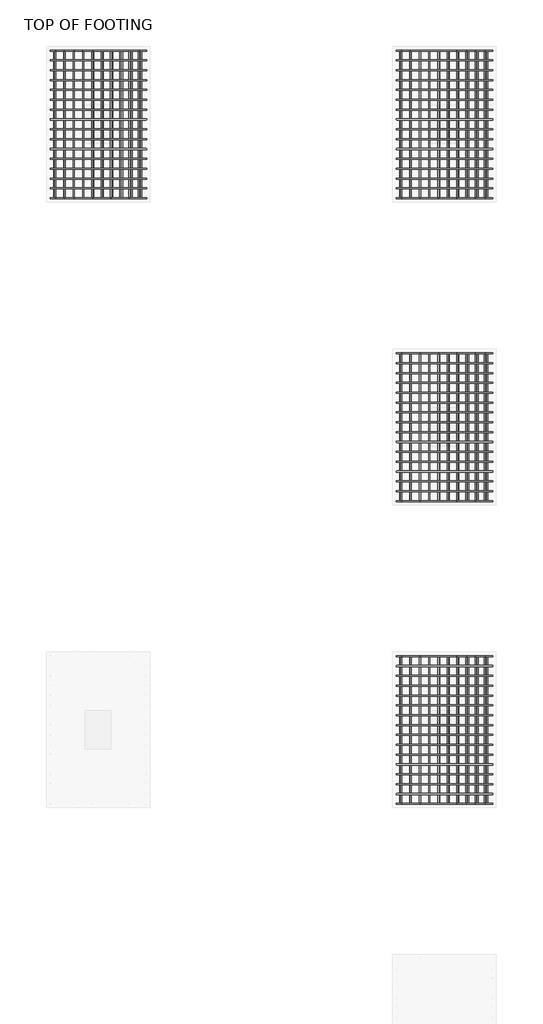
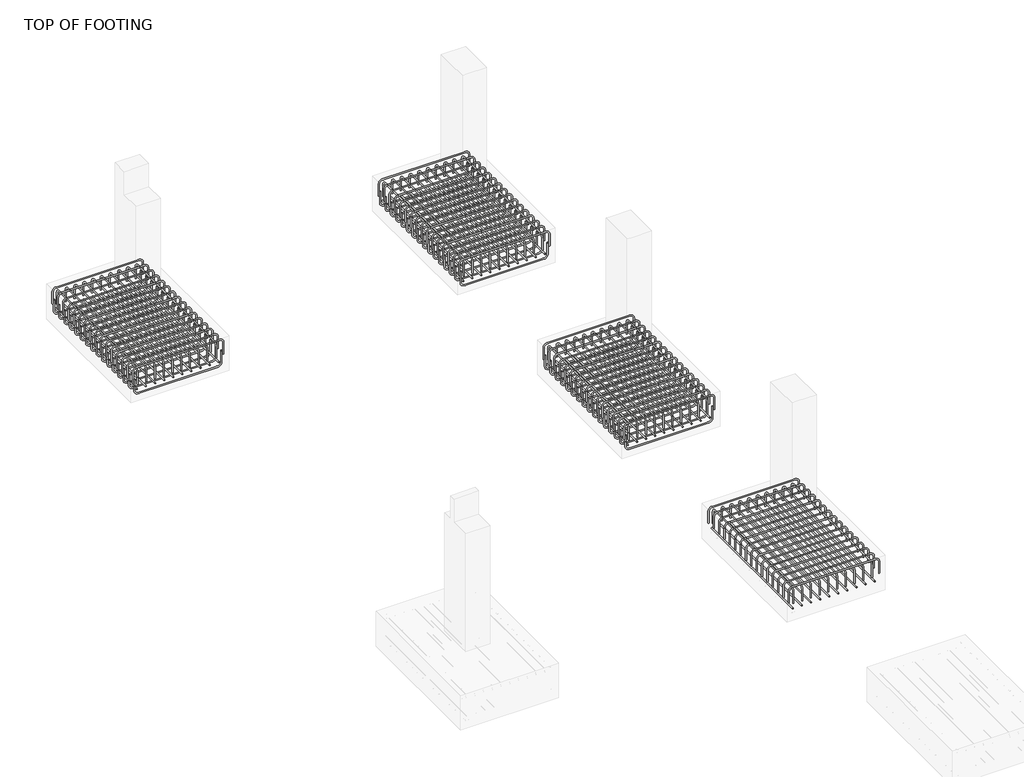
# One storey, part 8 of 8: 15 reinforcing bars.
"""IFC4 building model written with IfcOpenShell, lengths in millimetres."""

from ifc_helpers import new_model, si_unit, point, frame, origin, place, context, project, spatial, polyline, circle_curve, trimmed, segment, composite_curve, source, transform, mapped, element, save
from ifc_brep_helpers import swept_disk

model = new_model("IFC4")

# Units and contexts
model_context = context("Model", 3, world=origin())
ifc_project = project(units=[si_unit("LENGTHUNIT", "METRE", prefix="MILLI")], contexts=[model_context])

# Site, building, storey
site = spatial("IfcSite", under=ifc_project)
building = spatial("IfcBuilding", under=site)
storey = spatial("IfcBuildingStorey", under=building, Name="TOP OF FOOTING", Elevation=-1828.8)

# Reinforcing bars
placement = place(None, origin())
reinforcing_bar_shape = source(origin(), model_context, "Body", "SolidModel", [
    swept_disk(composite_curve([segment(polyline([(8698.4779803, 16626.3508557, -2021.4413313), (8698.4779803, 16626.3508557, -2168.7413313)]), True, "CONTINUOUS"), segment(trimmed(circle_curve(frame((8652.1279803, 16626.3508557, -2168.7413313), z_axis=(0.0, 1.0, 0.0), x_axis=(46.350000000000364, 0.0, 0.0)), 46.35), [point((8698.4779803, 16626.3508557, -2168.7413313))], [point((8652.1279803, 16626.3508557, -2215.0913313))], True, "CARTESIAN"), True, "CONTINUOUS"), segment(polyline([(8652.1279803, 16626.3508557, -2215.0913313), (7679.832969, 16626.3508557, -2215.0913313)]), True, "CONTINUOUS"), segment(trimmed(circle_curve(frame((7679.832969, 16626.3508557, -2168.7413313), z_axis=(0.0, 1.0, 0.0), x_axis=(0.0, 0.0, -46.34999999999991)), 46.35), [point((7679.832969, 16626.3508557, -2215.0913313))], [point((7633.482969, 16626.3508557, -2168.7413313))], True, "CARTESIAN"), True, "CONTINUOUS"), segment(polyline([(7633.482969, 16626.3508557, -2168.7413313), (7633.482969, 16626.3508557, -2021.4413313)]), True, "CONTINUOUS")], self_intersect=False), 6.35),
])
element("IfcReinforcingBar", 1, at=placement, inside=storey, context=model_context, shape_type="MappedRepresentation", body=[
    mapped(reinforcing_bar_shape, transform((0.0, 0.0, 0.0), x_axis=(1.0, 0.0, 0.0), y_axis=(0.0, 1.0, 0.0), z_axis=(0.0, 0.0, 1.0))),
    mapped(reinforcing_bar_shape, transform((0.0, -113.82, 0.0), x_axis=(1.0, 0.0, 0.0), y_axis=(0.0, 1.0, 0.0), z_axis=(0.0, 0.0, 1.0))),
    mapped(reinforcing_bar_shape, transform((0.0, -227.64, 0.0), x_axis=(1.0, 0.0, 0.0), y_axis=(0.0, 1.0, 0.0), z_axis=(0.0, 0.0, 1.0))),
    mapped(reinforcing_bar_shape, transform((0.0, -341.46, 0.0), x_axis=(1.0, 0.0, 0.0), y_axis=(0.0, 1.0, 0.0), z_axis=(0.0, 0.0, 1.0))),
    mapped(reinforcing_bar_shape, transform((0.0, -455.28, 0.0), x_axis=(1.0, 0.0, 0.0), y_axis=(0.0, 1.0, 0.0), z_axis=(0.0, 0.0, 1.0))),
    mapped(reinforcing_bar_shape, transform((0.0, -569.1, 0.0), x_axis=(1.0, 0.0, 0.0), y_axis=(0.0, 1.0, 0.0), z_axis=(0.0, 0.0, 1.0))),
    mapped(reinforcing_bar_shape, transform((0.0, -682.92, 0.0), x_axis=(1.0, 0.0, 0.0), y_axis=(0.0, 1.0, 0.0), z_axis=(0.0, 0.0, 1.0))),
    mapped(reinforcing_bar_shape, transform((0.0, -796.74, 0.0), x_axis=(1.0, 0.0, 0.0), y_axis=(0.0, 1.0, 0.0), z_axis=(0.0, 0.0, 1.0))),
    mapped(reinforcing_bar_shape, transform((0.0, -910.56, 0.0), x_axis=(1.0, 0.0, 0.0), y_axis=(0.0, 1.0, 0.0), z_axis=(0.0, 0.0, 1.0))),
    mapped(reinforcing_bar_shape, transform((0.0, -1024.38, 0.0), x_axis=(1.0, 0.0, 0.0), y_axis=(0.0, 1.0, 0.0), z_axis=(0.0, 0.0, 1.0))),
    mapped(reinforcing_bar_shape, transform((0.0, -1138.2, 0.0), x_axis=(1.0, 0.0, 0.0), y_axis=(0.0, 1.0, 0.0), z_axis=(0.0, 0.0, 1.0))),
    mapped(reinforcing_bar_shape, transform((0.0, -1252.02, 0.0), x_axis=(1.0, 0.0, 0.0), y_axis=(0.0, 1.0, 0.0), z_axis=(0.0, 0.0, 1.0))),
    mapped(reinforcing_bar_shape, transform((0.0, -1365.84, 0.0), x_axis=(1.0, 0.0, 0.0), y_axis=(0.0, 1.0, 0.0), z_axis=(0.0, 0.0, 1.0))),
    mapped(reinforcing_bar_shape, transform((0.0, -1479.66, 0.0), x_axis=(1.0, 0.0, 0.0), y_axis=(0.0, 1.0, 0.0), z_axis=(0.0, 0.0, 1.0))),
    mapped(reinforcing_bar_shape, transform((0.0, -1593.48, 0.0), x_axis=(1.0, 0.0, 0.0), y_axis=(0.0, 1.0, 0.0), z_axis=(0.0, 0.0, 1.0))),
    mapped(reinforcing_bar_shape, transform((0.0, -1707.3, 0.0), x_axis=(1.0, 0.0, 0.0), y_axis=(0.0, 1.0, 0.0), z_axis=(0.0, 0.0, 1.0))),
])
reinforcing_bar_2_shape = source(origin(), model_context, "Body", "SolidModel", [
    swept_disk(composite_curve([segment(polyline([(7615.6625983, 16626.3508557, -2068.8), (7615.6625983, 16626.3508557, -1921.5)]), True, "CONTINUOUS"), segment(trimmed(circle_curve(frame((7662.0125983, 16626.3508557, -1921.5), z_axis=(0.0, 1.0, 0.0), x_axis=(-46.349999999999454, 0.0, 0.0)), 46.35), [point((7615.6625983, 16626.3508557, -1921.5))], [point((7662.0125983, 16626.3508557, -1875.15))], True, "CARTESIAN"), True, "CONTINUOUS"), segment(polyline([(7662.0125983, 16626.3508557, -1875.15), (8676.6125983, 16626.3508557, -1875.15)]), True, "CONTINUOUS"), segment(trimmed(circle_curve(frame((8676.6125983, 16626.3508557, -1921.5), z_axis=(0.0, 1.0, 0.0), x_axis=(0.0, 0.0, 46.34999999999991)), 46.35), [point((8676.6125983, 16626.3508557, -1875.15))], [point((8722.9625983, 16626.3508557, -1921.5))], True, "CARTESIAN"), True, "CONTINUOUS"), segment(polyline([(8722.9625983, 16626.3508557, -1921.5), (8722.9625983, 16626.3508557, -2068.8)]), True, "CONTINUOUS")], self_intersect=False), 6.35),
])
element("IfcReinforcingBar", 2, at=placement, inside=storey, context=model_context, shape_type="MappedRepresentation", body=[
    mapped(reinforcing_bar_2_shape, transform((0.0, 0.0, 0.0), x_axis=(1.0, 0.0, 0.0), y_axis=(0.0, 1.0, 0.0), z_axis=(0.0, 0.0, 1.0))),
    mapped(reinforcing_bar_2_shape, transform((0.0, -113.82, 0.0), x_axis=(1.0, 0.0, 0.0), y_axis=(0.0, 1.0, 0.0), z_axis=(0.0, 0.0, 1.0))),
    mapped(reinforcing_bar_2_shape, transform((0.0, -227.64, 0.0), x_axis=(1.0, 0.0, 0.0), y_axis=(0.0, 1.0, 0.0), z_axis=(0.0, 0.0, 1.0))),
    mapped(reinforcing_bar_2_shape, transform((0.0, -341.46, 0.0), x_axis=(1.0, 0.0, 0.0), y_axis=(0.0, 1.0, 0.0), z_axis=(0.0, 0.0, 1.0))),
    mapped(reinforcing_bar_2_shape, transform((0.0, -455.28, 0.0), x_axis=(1.0, 0.0, 0.0), y_axis=(0.0, 1.0, 0.0), z_axis=(0.0, 0.0, 1.0))),
    mapped(reinforcing_bar_2_shape, transform((0.0, -569.1, 0.0), x_axis=(1.0, 0.0, 0.0), y_axis=(0.0, 1.0, 0.0), z_axis=(0.0, 0.0, 1.0))),
    mapped(reinforcing_bar_2_shape, transform((0.0, -682.92, 0.0), x_axis=(1.0, 0.0, 0.0), y_axis=(0.0, 1.0, 0.0), z_axis=(0.0, 0.0, 1.0))),
    mapped(reinforcing_bar_2_shape, transform((0.0, -796.74, 0.0), x_axis=(1.0, 0.0, 0.0), y_axis=(0.0, 1.0, 0.0), z_axis=(0.0, 0.0, 1.0))),
    mapped(reinforcing_bar_2_shape, transform((0.0, -910.56, 0.0), x_axis=(1.0, 0.0, 0.0), y_axis=(0.0, 1.0, 0.0), z_axis=(0.0, 0.0, 1.0))),
    mapped(reinforcing_bar_2_shape, transform((0.0, -1024.38, 0.0), x_axis=(1.0, 0.0, 0.0), y_axis=(0.0, 1.0, 0.0), z_axis=(0.0, 0.0, 1.0))),
    mapped(reinforcing_bar_2_shape, transform((0.0, -1138.2, 0.0), x_axis=(1.0, 0.0, 0.0), y_axis=(0.0, 1.0, 0.0), z_axis=(0.0, 0.0, 1.0))),
    mapped(reinforcing_bar_2_shape, transform((0.0, -1252.02, 0.0), x_axis=(1.0, 0.0, 0.0), y_axis=(0.0, 1.0, 0.0), z_axis=(0.0, 0.0, 1.0))),
    mapped(reinforcing_bar_2_shape, transform((0.0, -1365.84, 0.0), x_axis=(1.0, 0.0, 0.0), y_axis=(0.0, 1.0, 0.0), z_axis=(0.0, 0.0, 1.0))),
    mapped(reinforcing_bar_2_shape, transform((0.0, -1479.66, 0.0), x_axis=(1.0, 0.0, 0.0), y_axis=(0.0, 1.0, 0.0), z_axis=(0.0, 0.0, 1.0))),
    mapped(reinforcing_bar_2_shape, transform((0.0, -1593.48, 0.0), x_axis=(1.0, 0.0, 0.0), y_axis=(0.0, 1.0, 0.0), z_axis=(0.0, 0.0, 1.0))),
    mapped(reinforcing_bar_2_shape, transform((0.0, -1707.3, 0.0), x_axis=(1.0, 0.0, 0.0), y_axis=(0.0, 1.0, 0.0), z_axis=(0.0, 0.0, 1.0))),
])
reinforcing_bar_3_shape = source(origin(), model_context, "Body", "SolidModel", [
    swept_disk(composite_curve([segment(polyline([(7660.407291, 16632.7008557, -2155.1176129), (7660.407291, 14912.7008557, -2155.1176129)]), True, "CONTINUOUS")], self_intersect=False), 6.35),
])
element("IfcReinforcingBar", 3, at=placement, inside=storey, context=model_context, shape_type="MappedRepresentation", body=[
    mapped(reinforcing_bar_3_shape, transform((0.0, 0.0, 0.0), x_axis=(1.0, 0.0, 0.0), y_axis=(0.0, 1.0, 0.0), z_axis=(0.0, 0.0, 1.0))),
    mapped(reinforcing_bar_3_shape, transform((111.602188, 0.0, 0.0), x_axis=(1.0, 0.0, 0.0), y_axis=(0.0, 1.0, 0.0), z_axis=(0.0, 0.0, 1.0))),
    mapped(reinforcing_bar_3_shape, transform((223.2043759, 0.0, 0.0), x_axis=(1.0, 0.0, 0.0), y_axis=(0.0, 1.0, 0.0), z_axis=(0.0, 0.0, 1.0))),
    mapped(reinforcing_bar_3_shape, transform((334.8065639, 0.0, 0.0), x_axis=(1.0, 0.0, 0.0), y_axis=(0.0, 1.0, 0.0), z_axis=(0.0, 0.0, 1.0))),
    mapped(reinforcing_bar_3_shape, transform((446.4087519, 0.0, 0.0), x_axis=(1.0, 0.0, 0.0), y_axis=(0.0, 1.0, 0.0), z_axis=(0.0, 0.0, 1.0))),
    mapped(reinforcing_bar_3_shape, transform((558.0109398, 0.0, 0.0), x_axis=(1.0, 0.0, 0.0), y_axis=(0.0, 1.0, 0.0), z_axis=(0.0, 0.0, 1.0))),
    mapped(reinforcing_bar_3_shape, transform((669.6131278, 0.0, 0.0), x_axis=(1.0, 0.0, 0.0), y_axis=(0.0, 1.0, 0.0), z_axis=(0.0, 0.0, 1.0))),
    mapped(reinforcing_bar_3_shape, transform((781.2153158, 0.0, 0.0), x_axis=(1.0, 0.0, 0.0), y_axis=(0.0, 1.0, 0.0), z_axis=(0.0, 0.0, 1.0))),
    mapped(reinforcing_bar_3_shape, transform((892.8175037, 0.0, 0.0), x_axis=(1.0, 0.0, 0.0), y_axis=(0.0, 1.0, 0.0), z_axis=(0.0, 0.0, 1.0))),
    mapped(reinforcing_bar_3_shape, transform((1004.4196917, 0.0, 0.0), x_axis=(1.0, 0.0, 0.0), y_axis=(0.0, 1.0, 0.0), z_axis=(0.0, 0.0, 1.0))),
])
reinforcing_bar_4_shape = source(origin(), model_context, "Body", "SolidModel", [
    swept_disk(composite_curve([segment(polyline([(8635.7348019, 16626.3508557, -2094.6521303), (8635.7348019, 16626.3508557, -1947.3521303)]), True, "CONTINUOUS"), segment(trimmed(circle_curve(frame((8635.7348019, 16580.0008557, -1947.3521303), z_axis=(1.0, 0.0, 0.0), x_axis=(0.0, 46.349999999998545, 0.0)), 46.35), [point((8635.7348019, 16626.3508557, -1947.3521303))], [point((8635.7348019, 16580.0008557, -1901.0021303))], True, "CARTESIAN"), True, "CONTINUOUS"), segment(polyline([(8635.7348019, 16580.0008557, -1901.0021303), (8635.7348019, 14965.4008557, -1901.0021303)]), True, "CONTINUOUS"), segment(trimmed(circle_curve(frame((8635.7348019, 14965.4008557, -1947.3521303), z_axis=(1.0, 0.0, 0.0), x_axis=(0.0, 0.0, 46.34999999999991)), 46.35), [point((8635.7348019, 14965.4008557, -1901.0021303))], [point((8635.7348019, 14919.0508557, -1947.3521303))], True, "CARTESIAN"), True, "CONTINUOUS"), segment(polyline([(8635.7348019, 14919.0508557, -1947.3521303), (8635.7348019, 14919.0508557, -2094.6521303)]), True, "CONTINUOUS")], self_intersect=False), 6.35),
])
element("IfcReinforcingBar", 4, at=placement, inside=storey, context=model_context, shape_type="MappedRepresentation", body=[
    mapped(reinforcing_bar_4_shape, transform((0.0, 0.0, 0.0), x_axis=(1.0, 0.0, 0.0), y_axis=(0.0, 1.0, 0.0), z_axis=(0.0, 0.0, 1.0))),
    mapped(reinforcing_bar_4_shape, transform((-107.1680233, 0.0, 0.0), x_axis=(1.0, 0.0, 0.0), y_axis=(0.0, 1.0, 0.0), z_axis=(0.0, 0.0, 1.0))),
    mapped(reinforcing_bar_4_shape, transform((-214.3360466, 0.0, 0.0), x_axis=(1.0, 0.0, 0.0), y_axis=(0.0, 1.0, 0.0), z_axis=(0.0, 0.0, 1.0))),
    mapped(reinforcing_bar_4_shape, transform((-321.5040699, 0.0, 0.0), x_axis=(1.0, 0.0, 0.0), y_axis=(0.0, 1.0, 0.0), z_axis=(0.0, 0.0, 1.0))),
    mapped(reinforcing_bar_4_shape, transform((-428.6720932, 0.0, 0.0), x_axis=(1.0, 0.0, 0.0), y_axis=(0.0, 1.0, 0.0), z_axis=(0.0, 0.0, 1.0))),
    mapped(reinforcing_bar_4_shape, transform((-535.8401165, 0.0, 0.0), x_axis=(1.0, 0.0, 0.0), y_axis=(0.0, 1.0, 0.0), z_axis=(0.0, 0.0, 1.0))),
    mapped(reinforcing_bar_4_shape, transform((-643.0081398, 0.0, 0.0), x_axis=(1.0, 0.0, 0.0), y_axis=(0.0, 1.0, 0.0), z_axis=(0.0, 0.0, 1.0))),
    mapped(reinforcing_bar_4_shape, transform((-750.176163, 0.0, 0.0), x_axis=(1.0, 0.0, 0.0), y_axis=(0.0, 1.0, 0.0), z_axis=(0.0, 0.0, 1.0))),
    mapped(reinforcing_bar_4_shape, transform((-857.3441863, 0.0, 0.0), x_axis=(1.0, 0.0, 0.0), y_axis=(0.0, 1.0, 0.0), z_axis=(0.0, 0.0, 1.0))),
    mapped(reinforcing_bar_4_shape, transform((-964.5122096, 0.0, 0.0), x_axis=(1.0, 0.0, 0.0), y_axis=(0.0, 1.0, 0.0), z_axis=(0.0, 0.0, 1.0))),
])
reinforcing_bar_5_shape = source(origin(), model_context, "Body", "SolidModel", [
    swept_disk(composite_curve([segment(polyline([(12698.4779803, 16626.3508557, -2021.4413313), (12698.4779803, 16626.3508557, -2168.7413313)]), True, "CONTINUOUS"), segment(trimmed(circle_curve(frame((12652.1279803, 16626.3508557, -2168.7413313), z_axis=(0.0, 1.0, 0.0), x_axis=(46.350000000000364, 0.0, 0.0)), 46.35), [point((12698.4779803, 16626.3508557, -2168.7413313))], [point((12652.1279803, 16626.3508557, -2215.0913313))], True, "CARTESIAN"), True, "CONTINUOUS"), segment(polyline([(12652.1279803, 16626.3508557, -2215.0913313), (11679.832969, 16626.3508557, -2215.0913313)]), True, "CONTINUOUS"), segment(trimmed(circle_curve(frame((11679.832969, 16626.3508557, -2168.7413313), z_axis=(0.0, 1.0, 0.0), x_axis=(0.0, 0.0, -46.34999999999991)), 46.35), [point((11679.832969, 16626.3508557, -2215.0913313))], [point((11633.482969, 16626.3508557, -2168.7413313))], True, "CARTESIAN"), True, "CONTINUOUS"), segment(polyline([(11633.482969, 16626.3508557, -2168.7413313), (11633.482969, 16626.3508557, -2021.4413313)]), True, "CONTINUOUS")], self_intersect=False), 6.35),
])
element("IfcReinforcingBar", 5, at=placement, inside=storey, context=model_context, shape_type="MappedRepresentation", body=[
    mapped(reinforcing_bar_5_shape, transform((0.0, 0.0, 0.0), x_axis=(1.0, 0.0, 0.0), y_axis=(0.0, 1.0, 0.0), z_axis=(0.0, 0.0, 1.0))),
    mapped(reinforcing_bar_5_shape, transform((0.0, -113.82, 0.0), x_axis=(1.0, 0.0, 0.0), y_axis=(0.0, 1.0, 0.0), z_axis=(0.0, 0.0, 1.0))),
    mapped(reinforcing_bar_5_shape, transform((0.0, -227.64, 0.0), x_axis=(1.0, 0.0, 0.0), y_axis=(0.0, 1.0, 0.0), z_axis=(0.0, 0.0, 1.0))),
    mapped(reinforcing_bar_5_shape, transform((0.0, -341.46, 0.0), x_axis=(1.0, 0.0, 0.0), y_axis=(0.0, 1.0, 0.0), z_axis=(0.0, 0.0, 1.0))),
    mapped(reinforcing_bar_5_shape, transform((0.0, -455.28, 0.0), x_axis=(1.0, 0.0, 0.0), y_axis=(0.0, 1.0, 0.0), z_axis=(0.0, 0.0, 1.0))),
    mapped(reinforcing_bar_5_shape, transform((0.0, -569.1, 0.0), x_axis=(1.0, 0.0, 0.0), y_axis=(0.0, 1.0, 0.0), z_axis=(0.0, 0.0, 1.0))),
    mapped(reinforcing_bar_5_shape, transform((0.0, -682.92, 0.0), x_axis=(1.0, 0.0, 0.0), y_axis=(0.0, 1.0, 0.0), z_axis=(0.0, 0.0, 1.0))),
    mapped(reinforcing_bar_5_shape, transform((0.0, -796.74, 0.0), x_axis=(1.0, 0.0, 0.0), y_axis=(0.0, 1.0, 0.0), z_axis=(0.0, 0.0, 1.0))),
    mapped(reinforcing_bar_5_shape, transform((0.0, -910.56, 0.0), x_axis=(1.0, 0.0, 0.0), y_axis=(0.0, 1.0, 0.0), z_axis=(0.0, 0.0, 1.0))),
    mapped(reinforcing_bar_5_shape, transform((0.0, -1024.38, 0.0), x_axis=(1.0, 0.0, 0.0), y_axis=(0.0, 1.0, 0.0), z_axis=(0.0, 0.0, 1.0))),
    mapped(reinforcing_bar_5_shape, transform((0.0, -1138.2, 0.0), x_axis=(1.0, 0.0, 0.0), y_axis=(0.0, 1.0, 0.0), z_axis=(0.0, 0.0, 1.0))),
    mapped(reinforcing_bar_5_shape, transform((0.0, -1252.02, 0.0), x_axis=(1.0, 0.0, 0.0), y_axis=(0.0, 1.0, 0.0), z_axis=(0.0, 0.0, 1.0))),
    mapped(reinforcing_bar_5_shape, transform((0.0, -1365.84, 0.0), x_axis=(1.0, 0.0, 0.0), y_axis=(0.0, 1.0, 0.0), z_axis=(0.0, 0.0, 1.0))),
    mapped(reinforcing_bar_5_shape, transform((0.0, -1479.66, 0.0), x_axis=(1.0, 0.0, 0.0), y_axis=(0.0, 1.0, 0.0), z_axis=(0.0, 0.0, 1.0))),
    mapped(reinforcing_bar_5_shape, transform((0.0, -1593.48, 0.0), x_axis=(1.0, 0.0, 0.0), y_axis=(0.0, 1.0, 0.0), z_axis=(0.0, 0.0, 1.0))),
    mapped(reinforcing_bar_5_shape, transform((0.0, -1707.3, 0.0), x_axis=(1.0, 0.0, 0.0), y_axis=(0.0, 1.0, 0.0), z_axis=(0.0, 0.0, 1.0))),
])
reinforcing_bar_6_shape = source(origin(), model_context, "Body", "SolidModel", [
    swept_disk(composite_curve([segment(polyline([(11615.6625983, 16626.3508557, -2068.8), (11615.6625983, 16626.3508557, -1921.5)]), True, "CONTINUOUS"), segment(trimmed(circle_curve(frame((11662.0125983, 16626.3508557, -1921.5), z_axis=(0.0, 1.0, 0.0), x_axis=(-46.350000000000364, 0.0, 0.0)), 46.35), [point((11615.6625983, 16626.3508557, -1921.5))], [point((11662.0125983, 16626.3508557, -1875.15))], True, "CARTESIAN"), True, "CONTINUOUS"), segment(polyline([(11662.0125983, 16626.3508557, -1875.15), (12676.6125983, 16626.3508557, -1875.15)]), True, "CONTINUOUS"), segment(trimmed(circle_curve(frame((12676.6125983, 16626.3508557, -1921.5), z_axis=(0.0, 1.0, 0.0), x_axis=(0.0, 0.0, 46.34999999999991)), 46.35), [point((12676.6125983, 16626.3508557, -1875.15))], [point((12722.9625983, 16626.3508557, -1921.5))], True, "CARTESIAN"), True, "CONTINUOUS"), segment(polyline([(12722.9625983, 16626.3508557, -1921.5), (12722.9625983, 16626.3508557, -2068.8)]), True, "CONTINUOUS")], self_intersect=False), 6.35),
])
element("IfcReinforcingBar", 6, at=placement, inside=storey, context=model_context, shape_type="MappedRepresentation", body=[
    mapped(reinforcing_bar_6_shape, transform((0.0, 0.0, 0.0), x_axis=(1.0, 0.0, 0.0), y_axis=(0.0, 1.0, 0.0), z_axis=(0.0, 0.0, 1.0))),
    mapped(reinforcing_bar_6_shape, transform((0.0, -113.82, 0.0), x_axis=(1.0, 0.0, 0.0), y_axis=(0.0, 1.0, 0.0), z_axis=(0.0, 0.0, 1.0))),
    mapped(reinforcing_bar_6_shape, transform((0.0, -227.64, 0.0), x_axis=(1.0, 0.0, 0.0), y_axis=(0.0, 1.0, 0.0), z_axis=(0.0, 0.0, 1.0))),
    mapped(reinforcing_bar_6_shape, transform((0.0, -341.46, 0.0), x_axis=(1.0, 0.0, 0.0), y_axis=(0.0, 1.0, 0.0), z_axis=(0.0, 0.0, 1.0))),
    mapped(reinforcing_bar_6_shape, transform((0.0, -455.28, 0.0), x_axis=(1.0, 0.0, 0.0), y_axis=(0.0, 1.0, 0.0), z_axis=(0.0, 0.0, 1.0))),
    mapped(reinforcing_bar_6_shape, transform((0.0, -569.1, 0.0), x_axis=(1.0, 0.0, 0.0), y_axis=(0.0, 1.0, 0.0), z_axis=(0.0, 0.0, 1.0))),
    mapped(reinforcing_bar_6_shape, transform((0.0, -682.92, 0.0), x_axis=(1.0, 0.0, 0.0), y_axis=(0.0, 1.0, 0.0), z_axis=(0.0, 0.0, 1.0))),
    mapped(reinforcing_bar_6_shape, transform((0.0, -796.74, 0.0), x_axis=(1.0, 0.0, 0.0), y_axis=(0.0, 1.0, 0.0), z_axis=(0.0, 0.0, 1.0))),
    mapped(reinforcing_bar_6_shape, transform((0.0, -910.56, 0.0), x_axis=(1.0, 0.0, 0.0), y_axis=(0.0, 1.0, 0.0), z_axis=(0.0, 0.0, 1.0))),
    mapped(reinforcing_bar_6_shape, transform((0.0, -1024.38, 0.0), x_axis=(1.0, 0.0, 0.0), y_axis=(0.0, 1.0, 0.0), z_axis=(0.0, 0.0, 1.0))),
    mapped(reinforcing_bar_6_shape, transform((0.0, -1138.2, 0.0), x_axis=(1.0, 0.0, 0.0), y_axis=(0.0, 1.0, 0.0), z_axis=(0.0, 0.0, 1.0))),
    mapped(reinforcing_bar_6_shape, transform((0.0, -1252.02, 0.0), x_axis=(1.0, 0.0, 0.0), y_axis=(0.0, 1.0, 0.0), z_axis=(0.0, 0.0, 1.0))),
    mapped(reinforcing_bar_6_shape, transform((0.0, -1365.84, 0.0), x_axis=(1.0, 0.0, 0.0), y_axis=(0.0, 1.0, 0.0), z_axis=(0.0, 0.0, 1.0))),
    mapped(reinforcing_bar_6_shape, transform((0.0, -1479.66, 0.0), x_axis=(1.0, 0.0, 0.0), y_axis=(0.0, 1.0, 0.0), z_axis=(0.0, 0.0, 1.0))),
    mapped(reinforcing_bar_6_shape, transform((0.0, -1593.48, 0.0), x_axis=(1.0, 0.0, 0.0), y_axis=(0.0, 1.0, 0.0), z_axis=(0.0, 0.0, 1.0))),
    mapped(reinforcing_bar_6_shape, transform((0.0, -1707.3, 0.0), x_axis=(1.0, 0.0, 0.0), y_axis=(0.0, 1.0, 0.0), z_axis=(0.0, 0.0, 1.0))),
])
reinforcing_bar_7_shape = source(origin(), model_context, "Body", "SolidModel", [
    swept_disk(composite_curve([segment(polyline([(11660.407291, 16632.7008557, -2155.1176129), (11660.407291, 14912.7008557, -2155.1176129)]), True, "CONTINUOUS")], self_intersect=False), 6.35),
])
element("IfcReinforcingBar", 7, at=placement, inside=storey, context=model_context, shape_type="MappedRepresentation", body=[
    mapped(reinforcing_bar_7_shape, transform((0.0, 0.0, 0.0), x_axis=(1.0, 0.0, 0.0), y_axis=(0.0, 1.0, 0.0), z_axis=(0.0, 0.0, 1.0))),
    mapped(reinforcing_bar_7_shape, transform((111.602188, 0.0, 0.0), x_axis=(1.0, 0.0, 0.0), y_axis=(0.0, 1.0, 0.0), z_axis=(0.0, 0.0, 1.0))),
    mapped(reinforcing_bar_7_shape, transform((223.2043759, 0.0, 0.0), x_axis=(1.0, 0.0, 0.0), y_axis=(0.0, 1.0, 0.0), z_axis=(0.0, 0.0, 1.0))),
    mapped(reinforcing_bar_7_shape, transform((334.8065639, 0.0, 0.0), x_axis=(1.0, 0.0, 0.0), y_axis=(0.0, 1.0, 0.0), z_axis=(0.0, 0.0, 1.0))),
    mapped(reinforcing_bar_7_shape, transform((446.4087519, 0.0, 0.0), x_axis=(1.0, 0.0, 0.0), y_axis=(0.0, 1.0, 0.0), z_axis=(0.0, 0.0, 1.0))),
    mapped(reinforcing_bar_7_shape, transform((558.0109398, 0.0, 0.0), x_axis=(1.0, 0.0, 0.0), y_axis=(0.0, 1.0, 0.0), z_axis=(0.0, 0.0, 1.0))),
    mapped(reinforcing_bar_7_shape, transform((669.6131278, 0.0, 0.0), x_axis=(1.0, 0.0, 0.0), y_axis=(0.0, 1.0, 0.0), z_axis=(0.0, 0.0, 1.0))),
    mapped(reinforcing_bar_7_shape, transform((781.2153158, 0.0, 0.0), x_axis=(1.0, 0.0, 0.0), y_axis=(0.0, 1.0, 0.0), z_axis=(0.0, 0.0, 1.0))),
    mapped(reinforcing_bar_7_shape, transform((892.8175037, 0.0, 0.0), x_axis=(1.0, 0.0, 0.0), y_axis=(0.0, 1.0, 0.0), z_axis=(0.0, 0.0, 1.0))),
    mapped(reinforcing_bar_7_shape, transform((1004.4196917, 0.0, 0.0), x_axis=(1.0, 0.0, 0.0), y_axis=(0.0, 1.0, 0.0), z_axis=(0.0, 0.0, 1.0))),
])
reinforcing_bar_8_shape = source(origin(), model_context, "Body", "SolidModel", [
    swept_disk(composite_curve([segment(polyline([(12635.7348019, 16626.3508557, -2094.6521303), (12635.7348019, 16626.3508557, -1947.3521303)]), True, "CONTINUOUS"), segment(trimmed(circle_curve(frame((12635.7348019, 16580.0008557, -1947.3521303), z_axis=(1.0, 0.0, 0.0), x_axis=(0.0, 46.349999999998545, 0.0)), 46.35), [point((12635.7348019, 16626.3508557, -1947.3521303))], [point((12635.7348019, 16580.0008557, -1901.0021303))], True, "CARTESIAN"), True, "CONTINUOUS"), segment(polyline([(12635.7348019, 16580.0008557, -1901.0021303), (12635.7348019, 14965.4008557, -1901.0021303)]), True, "CONTINUOUS"), segment(trimmed(circle_curve(frame((12635.7348019, 14965.4008557, -1947.3521303), z_axis=(1.0, 0.0, 0.0), x_axis=(0.0, 0.0, 46.34999999999991)), 46.35), [point((12635.7348019, 14965.4008557, -1901.0021303))], [point((12635.7348019, 14919.0508557, -1947.3521303))], True, "CARTESIAN"), True, "CONTINUOUS"), segment(polyline([(12635.7348019, 14919.0508557, -1947.3521303), (12635.7348019, 14919.0508557, -2094.6521303)]), True, "CONTINUOUS")], self_intersect=False), 6.35),
])
element("IfcReinforcingBar", 8, at=placement, inside=storey, context=model_context, shape_type="MappedRepresentation", body=[
    mapped(reinforcing_bar_8_shape, transform((0.0, 0.0, 0.0), x_axis=(1.0, 0.0, 0.0), y_axis=(0.0, 1.0, 0.0), z_axis=(0.0, 0.0, 1.0))),
    mapped(reinforcing_bar_8_shape, transform((-107.1680233, 0.0, 0.0), x_axis=(1.0, 0.0, 0.0), y_axis=(0.0, 1.0, 0.0), z_axis=(0.0, 0.0, 1.0))),
    mapped(reinforcing_bar_8_shape, transform((-214.3360466, 0.0, 0.0), x_axis=(1.0, 0.0, 0.0), y_axis=(0.0, 1.0, 0.0), z_axis=(0.0, 0.0, 1.0))),
    mapped(reinforcing_bar_8_shape, transform((-321.5040699, 0.0, 0.0), x_axis=(1.0, 0.0, 0.0), y_axis=(0.0, 1.0, 0.0), z_axis=(0.0, 0.0, 1.0))),
    mapped(reinforcing_bar_8_shape, transform((-428.6720932, 0.0, 0.0), x_axis=(1.0, 0.0, 0.0), y_axis=(0.0, 1.0, 0.0), z_axis=(0.0, 0.0, 1.0))),
    mapped(reinforcing_bar_8_shape, transform((-535.8401165, 0.0, 0.0), x_axis=(1.0, 0.0, 0.0), y_axis=(0.0, 1.0, 0.0), z_axis=(0.0, 0.0, 1.0))),
    mapped(reinforcing_bar_8_shape, transform((-643.0081398, 0.0, 0.0), x_axis=(1.0, 0.0, 0.0), y_axis=(0.0, 1.0, 0.0), z_axis=(0.0, 0.0, 1.0))),
    mapped(reinforcing_bar_8_shape, transform((-750.176163, 0.0, 0.0), x_axis=(1.0, 0.0, 0.0), y_axis=(0.0, 1.0, 0.0), z_axis=(0.0, 0.0, 1.0))),
    mapped(reinforcing_bar_8_shape, transform((-857.3441863, 0.0, 0.0), x_axis=(1.0, 0.0, 0.0), y_axis=(0.0, 1.0, 0.0), z_axis=(0.0, 0.0, 1.0))),
    mapped(reinforcing_bar_8_shape, transform((-964.5122096, 0.0, 0.0), x_axis=(1.0, 0.0, 0.0), y_axis=(0.0, 1.0, 0.0), z_axis=(0.0, 0.0, 1.0))),
])
reinforcing_bar_9_shape = source(origin(), model_context, "Body", "SolidModel", [
    swept_disk(composite_curve([segment(polyline([(12698.4779803, 13126.3508557, -2021.4413313), (12698.4779803, 13126.3508557, -2168.7413313)]), True, "CONTINUOUS"), segment(trimmed(circle_curve(frame((12652.1279803, 13126.3508557, -2168.7413313), z_axis=(0.0, 1.0, 0.0), x_axis=(46.350000000000364, 0.0, 0.0)), 46.35), [point((12698.4779803, 13126.3508557, -2168.7413313))], [point((12652.1279803, 13126.3508557, -2215.0913313))], True, "CARTESIAN"), True, "CONTINUOUS"), segment(polyline([(12652.1279803, 13126.3508557, -2215.0913313), (11679.832969, 13126.3508557, -2215.0913313)]), True, "CONTINUOUS"), segment(trimmed(circle_curve(frame((11679.832969, 13126.3508557, -2168.7413313), z_axis=(0.0, 1.0, 0.0), x_axis=(0.0, 0.0, -46.34999999999991)), 46.35), [point((11679.832969, 13126.3508557, -2215.0913313))], [point((11633.482969, 13126.3508557, -2168.7413313))], True, "CARTESIAN"), True, "CONTINUOUS"), segment(polyline([(11633.482969, 13126.3508557, -2168.7413313), (11633.482969, 13126.3508557, -2021.4413313)]), True, "CONTINUOUS")], self_intersect=False), 6.35),
])
element("IfcReinforcingBar", 9, at=placement, inside=storey, context=model_context, shape_type="MappedRepresentation", body=[
    mapped(reinforcing_bar_9_shape, transform((0.0, 0.0, 0.0), x_axis=(1.0, 0.0, 0.0), y_axis=(0.0, 1.0, 0.0), z_axis=(0.0, 0.0, 1.0))),
    mapped(reinforcing_bar_9_shape, transform((0.0, -113.82, 0.0), x_axis=(1.0, 0.0, 0.0), y_axis=(0.0, 1.0, 0.0), z_axis=(0.0, 0.0, 1.0))),
    mapped(reinforcing_bar_9_shape, transform((0.0, -227.64, 0.0), x_axis=(1.0, 0.0, 0.0), y_axis=(0.0, 1.0, 0.0), z_axis=(0.0, 0.0, 1.0))),
    mapped(reinforcing_bar_9_shape, transform((0.0, -341.46, 0.0), x_axis=(1.0, 0.0, 0.0), y_axis=(0.0, 1.0, 0.0), z_axis=(0.0, 0.0, 1.0))),
    mapped(reinforcing_bar_9_shape, transform((0.0, -455.28, 0.0), x_axis=(1.0, 0.0, 0.0), y_axis=(0.0, 1.0, 0.0), z_axis=(0.0, 0.0, 1.0))),
    mapped(reinforcing_bar_9_shape, transform((0.0, -569.1, 0.0), x_axis=(1.0, 0.0, 0.0), y_axis=(0.0, 1.0, 0.0), z_axis=(0.0, 0.0, 1.0))),
    mapped(reinforcing_bar_9_shape, transform((0.0, -682.92, 0.0), x_axis=(1.0, 0.0, 0.0), y_axis=(0.0, 1.0, 0.0), z_axis=(0.0, 0.0, 1.0))),
    mapped(reinforcing_bar_9_shape, transform((0.0, -796.74, 0.0), x_axis=(1.0, 0.0, 0.0), y_axis=(0.0, 1.0, 0.0), z_axis=(0.0, 0.0, 1.0))),
    mapped(reinforcing_bar_9_shape, transform((0.0, -910.56, 0.0), x_axis=(1.0, 0.0, 0.0), y_axis=(0.0, 1.0, 0.0), z_axis=(0.0, 0.0, 1.0))),
    mapped(reinforcing_bar_9_shape, transform((0.0, -1024.38, 0.0), x_axis=(1.0, 0.0, 0.0), y_axis=(0.0, 1.0, 0.0), z_axis=(0.0, 0.0, 1.0))),
    mapped(reinforcing_bar_9_shape, transform((0.0, -1138.2, 0.0), x_axis=(1.0, 0.0, 0.0), y_axis=(0.0, 1.0, 0.0), z_axis=(0.0, 0.0, 1.0))),
    mapped(reinforcing_bar_9_shape, transform((0.0, -1252.02, 0.0), x_axis=(1.0, 0.0, 0.0), y_axis=(0.0, 1.0, 0.0), z_axis=(0.0, 0.0, 1.0))),
    mapped(reinforcing_bar_9_shape, transform((0.0, -1365.84, 0.0), x_axis=(1.0, 0.0, 0.0), y_axis=(0.0, 1.0, 0.0), z_axis=(0.0, 0.0, 1.0))),
    mapped(reinforcing_bar_9_shape, transform((0.0, -1479.66, 0.0), x_axis=(1.0, 0.0, 0.0), y_axis=(0.0, 1.0, 0.0), z_axis=(0.0, 0.0, 1.0))),
    mapped(reinforcing_bar_9_shape, transform((0.0, -1593.48, 0.0), x_axis=(1.0, 0.0, 0.0), y_axis=(0.0, 1.0, 0.0), z_axis=(0.0, 0.0, 1.0))),
    mapped(reinforcing_bar_9_shape, transform((0.0, -1707.3, 0.0), x_axis=(1.0, 0.0, 0.0), y_axis=(0.0, 1.0, 0.0), z_axis=(0.0, 0.0, 1.0))),
])
reinforcing_bar_10_shape = source(origin(), model_context, "Body", "SolidModel", [
    swept_disk(composite_curve([segment(polyline([(11615.6625983, 13126.3508557, -2068.8), (11615.6625983, 13126.3508557, -1921.5)]), True, "CONTINUOUS"), segment(trimmed(circle_curve(frame((11662.0125983, 13126.3508557, -1921.5), z_axis=(0.0, 1.0, 0.0), x_axis=(-46.350000000000364, 0.0, 0.0)), 46.35), [point((11615.6625983, 13126.3508557, -1921.5))], [point((11662.0125983, 13126.3508557, -1875.15))], True, "CARTESIAN"), True, "CONTINUOUS"), segment(polyline([(11662.0125983, 13126.3508557, -1875.15), (12676.6125983, 13126.3508557, -1875.15)]), True, "CONTINUOUS"), segment(trimmed(circle_curve(frame((12676.6125983, 13126.3508557, -1921.5), z_axis=(0.0, 1.0, 0.0), x_axis=(0.0, 0.0, 46.34999999999991)), 46.35), [point((12676.6125983, 13126.3508557, -1875.15))], [point((12722.9625983, 13126.3508557, -1921.5))], True, "CARTESIAN"), True, "CONTINUOUS"), segment(polyline([(12722.9625983, 13126.3508557, -1921.5), (12722.9625983, 13126.3508557, -2068.8)]), True, "CONTINUOUS")], self_intersect=False), 6.35),
])
element("IfcReinforcingBar", 10, at=placement, inside=storey, context=model_context, shape_type="MappedRepresentation", body=[
    mapped(reinforcing_bar_10_shape, transform((0.0, 0.0, 0.0), x_axis=(1.0, 0.0, 0.0), y_axis=(0.0, 1.0, 0.0), z_axis=(0.0, 0.0, 1.0))),
    mapped(reinforcing_bar_10_shape, transform((0.0, -113.82, 0.0), x_axis=(1.0, 0.0, 0.0), y_axis=(0.0, 1.0, 0.0), z_axis=(0.0, 0.0, 1.0))),
    mapped(reinforcing_bar_10_shape, transform((0.0, -227.64, 0.0), x_axis=(1.0, 0.0, 0.0), y_axis=(0.0, 1.0, 0.0), z_axis=(0.0, 0.0, 1.0))),
    mapped(reinforcing_bar_10_shape, transform((0.0, -341.46, 0.0), x_axis=(1.0, 0.0, 0.0), y_axis=(0.0, 1.0, 0.0), z_axis=(0.0, 0.0, 1.0))),
    mapped(reinforcing_bar_10_shape, transform((0.0, -455.28, 0.0), x_axis=(1.0, 0.0, 0.0), y_axis=(0.0, 1.0, 0.0), z_axis=(0.0, 0.0, 1.0))),
    mapped(reinforcing_bar_10_shape, transform((0.0, -569.1, 0.0), x_axis=(1.0, 0.0, 0.0), y_axis=(0.0, 1.0, 0.0), z_axis=(0.0, 0.0, 1.0))),
    mapped(reinforcing_bar_10_shape, transform((0.0, -682.92, 0.0), x_axis=(1.0, 0.0, 0.0), y_axis=(0.0, 1.0, 0.0), z_axis=(0.0, 0.0, 1.0))),
    mapped(reinforcing_bar_10_shape, transform((0.0, -796.74, 0.0), x_axis=(1.0, 0.0, 0.0), y_axis=(0.0, 1.0, 0.0), z_axis=(0.0, 0.0, 1.0))),
    mapped(reinforcing_bar_10_shape, transform((0.0, -910.56, 0.0), x_axis=(1.0, 0.0, 0.0), y_axis=(0.0, 1.0, 0.0), z_axis=(0.0, 0.0, 1.0))),
    mapped(reinforcing_bar_10_shape, transform((0.0, -1024.38, 0.0), x_axis=(1.0, 0.0, 0.0), y_axis=(0.0, 1.0, 0.0), z_axis=(0.0, 0.0, 1.0))),
    mapped(reinforcing_bar_10_shape, transform((0.0, -1138.2, 0.0), x_axis=(1.0, 0.0, 0.0), y_axis=(0.0, 1.0, 0.0), z_axis=(0.0, 0.0, 1.0))),
    mapped(reinforcing_bar_10_shape, transform((0.0, -1252.02, 0.0), x_axis=(1.0, 0.0, 0.0), y_axis=(0.0, 1.0, 0.0), z_axis=(0.0, 0.0, 1.0))),
    mapped(reinforcing_bar_10_shape, transform((0.0, -1365.84, 0.0), x_axis=(1.0, 0.0, 0.0), y_axis=(0.0, 1.0, 0.0), z_axis=(0.0, 0.0, 1.0))),
    mapped(reinforcing_bar_10_shape, transform((0.0, -1479.66, 0.0), x_axis=(1.0, 0.0, 0.0), y_axis=(0.0, 1.0, 0.0), z_axis=(0.0, 0.0, 1.0))),
    mapped(reinforcing_bar_10_shape, transform((0.0, -1593.48, 0.0), x_axis=(1.0, 0.0, 0.0), y_axis=(0.0, 1.0, 0.0), z_axis=(0.0, 0.0, 1.0))),
    mapped(reinforcing_bar_10_shape, transform((0.0, -1707.3, 0.0), x_axis=(1.0, 0.0, 0.0), y_axis=(0.0, 1.0, 0.0), z_axis=(0.0, 0.0, 1.0))),
])
reinforcing_bar_11_shape = source(origin(), model_context, "Body", "SolidModel", [
    swept_disk(composite_curve([segment(polyline([(11660.407291, 13132.7008557, -2155.1176129), (11660.407291, 11412.7008557, -2155.1176129)]), True, "CONTINUOUS")], self_intersect=False), 6.35),
])
element("IfcReinforcingBar", 11, at=placement, inside=storey, context=model_context, shape_type="MappedRepresentation", body=[
    mapped(reinforcing_bar_11_shape, transform((0.0, 0.0, 0.0), x_axis=(1.0, 0.0, 0.0), y_axis=(0.0, 1.0, 0.0), z_axis=(0.0, 0.0, 1.0))),
    mapped(reinforcing_bar_11_shape, transform((111.602188, 0.0, 0.0), x_axis=(1.0, 0.0, 0.0), y_axis=(0.0, 1.0, 0.0), z_axis=(0.0, 0.0, 1.0))),
    mapped(reinforcing_bar_11_shape, transform((223.2043759, 0.0, 0.0), x_axis=(1.0, 0.0, 0.0), y_axis=(0.0, 1.0, 0.0), z_axis=(0.0, 0.0, 1.0))),
    mapped(reinforcing_bar_11_shape, transform((334.8065639, 0.0, 0.0), x_axis=(1.0, 0.0, 0.0), y_axis=(0.0, 1.0, 0.0), z_axis=(0.0, 0.0, 1.0))),
    mapped(reinforcing_bar_11_shape, transform((446.4087519, 0.0, 0.0), x_axis=(1.0, 0.0, 0.0), y_axis=(0.0, 1.0, 0.0), z_axis=(0.0, 0.0, 1.0))),
    mapped(reinforcing_bar_11_shape, transform((558.0109398, 0.0, 0.0), x_axis=(1.0, 0.0, 0.0), y_axis=(0.0, 1.0, 0.0), z_axis=(0.0, 0.0, 1.0))),
    mapped(reinforcing_bar_11_shape, transform((669.6131278, 0.0, 0.0), x_axis=(1.0, 0.0, 0.0), y_axis=(0.0, 1.0, 0.0), z_axis=(0.0, 0.0, 1.0))),
    mapped(reinforcing_bar_11_shape, transform((781.2153158, 0.0, 0.0), x_axis=(1.0, 0.0, 0.0), y_axis=(0.0, 1.0, 0.0), z_axis=(0.0, 0.0, 1.0))),
    mapped(reinforcing_bar_11_shape, transform((892.8175037, 0.0, 0.0), x_axis=(1.0, 0.0, 0.0), y_axis=(0.0, 1.0, 0.0), z_axis=(0.0, 0.0, 1.0))),
    mapped(reinforcing_bar_11_shape, transform((1004.4196917, 0.0, 0.0), x_axis=(1.0, 0.0, 0.0), y_axis=(0.0, 1.0, 0.0), z_axis=(0.0, 0.0, 1.0))),
])
reinforcing_bar_12_shape = source(origin(), model_context, "Body", "SolidModel", [
    swept_disk(composite_curve([segment(polyline([(12635.7348019, 13126.3508557, -2094.6521303), (12635.7348019, 13126.3508557, -1947.3521303)]), True, "CONTINUOUS"), segment(trimmed(circle_curve(frame((12635.7348019, 13080.0008557, -1947.3521303), z_axis=(1.0, 0.0, 0.0), x_axis=(0.0, 46.350000000000364, 0.0)), 46.35), [point((12635.7348019, 13126.3508557, -1947.3521303))], [point((12635.7348019, 13080.0008557, -1901.0021303))], True, "CARTESIAN"), True, "CONTINUOUS"), segment(polyline([(12635.7348019, 13080.0008557, -1901.0021303), (12635.7348019, 11465.4008557, -1901.0021303)]), True, "CONTINUOUS"), segment(trimmed(circle_curve(frame((12635.7348019, 11465.4008557, -1947.3521303), z_axis=(1.0, 0.0, 0.0), x_axis=(0.0, 0.0, 46.34999999999991)), 46.35), [point((12635.7348019, 11465.4008557, -1901.0021303))], [point((12635.7348019, 11419.0508557, -1947.3521303))], True, "CARTESIAN"), True, "CONTINUOUS"), segment(polyline([(12635.7348019, 11419.0508557, -1947.3521303), (12635.7348019, 11419.0508557, -2094.6521303)]), True, "CONTINUOUS")], self_intersect=False), 6.35),
])
element("IfcReinforcingBar", 12, at=placement, inside=storey, context=model_context, shape_type="MappedRepresentation", body=[
    mapped(reinforcing_bar_12_shape, transform((0.0, 0.0, 0.0), x_axis=(1.0, 0.0, 0.0), y_axis=(0.0, 1.0, 0.0), z_axis=(0.0, 0.0, 1.0))),
    mapped(reinforcing_bar_12_shape, transform((-107.1680233, 0.0, 0.0), x_axis=(1.0, 0.0, 0.0), y_axis=(0.0, 1.0, 0.0), z_axis=(0.0, 0.0, 1.0))),
    mapped(reinforcing_bar_12_shape, transform((-214.3360466, 0.0, 0.0), x_axis=(1.0, 0.0, 0.0), y_axis=(0.0, 1.0, 0.0), z_axis=(0.0, 0.0, 1.0))),
    mapped(reinforcing_bar_12_shape, transform((-321.5040699, 0.0, 0.0), x_axis=(1.0, 0.0, 0.0), y_axis=(0.0, 1.0, 0.0), z_axis=(0.0, 0.0, 1.0))),
    mapped(reinforcing_bar_12_shape, transform((-428.6720932, 0.0, 0.0), x_axis=(1.0, 0.0, 0.0), y_axis=(0.0, 1.0, 0.0), z_axis=(0.0, 0.0, 1.0))),
    mapped(reinforcing_bar_12_shape, transform((-535.8401165, 0.0, 0.0), x_axis=(1.0, 0.0, 0.0), y_axis=(0.0, 1.0, 0.0), z_axis=(0.0, 0.0, 1.0))),
    mapped(reinforcing_bar_12_shape, transform((-643.0081398, 0.0, 0.0), x_axis=(1.0, 0.0, 0.0), y_axis=(0.0, 1.0, 0.0), z_axis=(0.0, 0.0, 1.0))),
    mapped(reinforcing_bar_12_shape, transform((-750.176163, 0.0, 0.0), x_axis=(1.0, 0.0, 0.0), y_axis=(0.0, 1.0, 0.0), z_axis=(0.0, 0.0, 1.0))),
    mapped(reinforcing_bar_12_shape, transform((-857.3441863, 0.0, 0.0), x_axis=(1.0, 0.0, 0.0), y_axis=(0.0, 1.0, 0.0), z_axis=(0.0, 0.0, 1.0))),
    mapped(reinforcing_bar_12_shape, transform((-964.5122096, 0.0, 0.0), x_axis=(1.0, 0.0, 0.0), y_axis=(0.0, 1.0, 0.0), z_axis=(0.0, 0.0, 1.0))),
])
reinforcing_bar_13_shape = source(origin(), model_context, "Body", "SolidModel", [
    swept_disk(composite_curve([segment(polyline([(11615.6625983, 9626.3508557, -2068.8), (11615.6625983, 9626.3508557, -1921.5)]), True, "CONTINUOUS"), segment(trimmed(circle_curve(frame((11662.0125983, 9626.3508557, -1921.5), z_axis=(0.0, 1.0, 0.0), x_axis=(-46.350000000000364, 0.0, 0.0)), 46.35), [point((11615.6625983, 9626.3508557, -1921.5))], [point((11662.0125983, 9626.3508557, -1875.15))], True, "CARTESIAN"), True, "CONTINUOUS"), segment(polyline([(11662.0125983, 9626.3508557, -1875.15), (12676.6125983, 9626.3508557, -1875.15)]), True, "CONTINUOUS"), segment(trimmed(circle_curve(frame((12676.6125983, 9626.3508557, -1921.5), z_axis=(0.0, 1.0, 0.0), x_axis=(0.0, 0.0, 46.34999999999991)), 46.35), [point((12676.6125983, 9626.3508557, -1875.15))], [point((12722.9625983, 9626.3508557, -1921.5))], True, "CARTESIAN"), True, "CONTINUOUS"), segment(polyline([(12722.9625983, 9626.3508557, -1921.5), (12722.9625983, 9626.3508557, -2068.8)]), True, "CONTINUOUS")], self_intersect=False), 6.35),
])
element("IfcReinforcingBar", 13, at=placement, inside=storey, context=model_context, shape_type="MappedRepresentation", body=[
    mapped(reinforcing_bar_13_shape, transform((0.0, 0.0, 0.0), x_axis=(1.0, 0.0, 0.0), y_axis=(0.0, 1.0, 0.0), z_axis=(0.0, 0.0, 1.0))),
    mapped(reinforcing_bar_13_shape, transform((0.0, -113.82, 0.0), x_axis=(1.0, 0.0, 0.0), y_axis=(0.0, 1.0, 0.0), z_axis=(0.0, 0.0, 1.0))),
    mapped(reinforcing_bar_13_shape, transform((0.0, -227.64, 0.0), x_axis=(1.0, 0.0, 0.0), y_axis=(0.0, 1.0, 0.0), z_axis=(0.0, 0.0, 1.0))),
    mapped(reinforcing_bar_13_shape, transform((0.0, -341.46, 0.0), x_axis=(1.0, 0.0, 0.0), y_axis=(0.0, 1.0, 0.0), z_axis=(0.0, 0.0, 1.0))),
    mapped(reinforcing_bar_13_shape, transform((0.0, -455.28, 0.0), x_axis=(1.0, 0.0, 0.0), y_axis=(0.0, 1.0, 0.0), z_axis=(0.0, 0.0, 1.0))),
    mapped(reinforcing_bar_13_shape, transform((0.0, -569.1, 0.0), x_axis=(1.0, 0.0, 0.0), y_axis=(0.0, 1.0, 0.0), z_axis=(0.0, 0.0, 1.0))),
    mapped(reinforcing_bar_13_shape, transform((0.0, -682.92, 0.0), x_axis=(1.0, 0.0, 0.0), y_axis=(0.0, 1.0, 0.0), z_axis=(0.0, 0.0, 1.0))),
    mapped(reinforcing_bar_13_shape, transform((0.0, -796.74, 0.0), x_axis=(1.0, 0.0, 0.0), y_axis=(0.0, 1.0, 0.0), z_axis=(0.0, 0.0, 1.0))),
    mapped(reinforcing_bar_13_shape, transform((0.0, -910.56, 0.0), x_axis=(1.0, 0.0, 0.0), y_axis=(0.0, 1.0, 0.0), z_axis=(0.0, 0.0, 1.0))),
    mapped(reinforcing_bar_13_shape, transform((0.0, -1024.38, 0.0), x_axis=(1.0, 0.0, 0.0), y_axis=(0.0, 1.0, 0.0), z_axis=(0.0, 0.0, 1.0))),
    mapped(reinforcing_bar_13_shape, transform((0.0, -1138.2, 0.0), x_axis=(1.0, 0.0, 0.0), y_axis=(0.0, 1.0, 0.0), z_axis=(0.0, 0.0, 1.0))),
    mapped(reinforcing_bar_13_shape, transform((0.0, -1252.02, 0.0), x_axis=(1.0, 0.0, 0.0), y_axis=(0.0, 1.0, 0.0), z_axis=(0.0, 0.0, 1.0))),
    mapped(reinforcing_bar_13_shape, transform((0.0, -1365.84, 0.0), x_axis=(1.0, 0.0, 0.0), y_axis=(0.0, 1.0, 0.0), z_axis=(0.0, 0.0, 1.0))),
    mapped(reinforcing_bar_13_shape, transform((0.0, -1479.66, 0.0), x_axis=(1.0, 0.0, 0.0), y_axis=(0.0, 1.0, 0.0), z_axis=(0.0, 0.0, 1.0))),
    mapped(reinforcing_bar_13_shape, transform((0.0, -1593.48, 0.0), x_axis=(1.0, 0.0, 0.0), y_axis=(0.0, 1.0, 0.0), z_axis=(0.0, 0.0, 1.0))),
    mapped(reinforcing_bar_13_shape, transform((0.0, -1707.3, 0.0), x_axis=(1.0, 0.0, 0.0), y_axis=(0.0, 1.0, 0.0), z_axis=(0.0, 0.0, 1.0))),
])
reinforcing_bar_14_shape = source(origin(), model_context, "Body", "SolidModel", [
    swept_disk(composite_curve([segment(polyline([(11660.407291, 9632.7008557, -2155.1176129), (11660.407291, 7912.7008557, -2155.1176129)]), True, "CONTINUOUS")], self_intersect=False), 6.35),
])
element("IfcReinforcingBar", 14, at=placement, inside=storey, context=model_context, shape_type="MappedRepresentation", body=[
    mapped(reinforcing_bar_14_shape, transform((0.0, 0.0, 0.0), x_axis=(1.0, 0.0, 0.0), y_axis=(0.0, 1.0, 0.0), z_axis=(0.0, 0.0, 1.0))),
    mapped(reinforcing_bar_14_shape, transform((111.602188, 0.0, 0.0), x_axis=(1.0, 0.0, 0.0), y_axis=(0.0, 1.0, 0.0), z_axis=(0.0, 0.0, 1.0))),
    mapped(reinforcing_bar_14_shape, transform((223.2043759, 0.0, 0.0), x_axis=(1.0, 0.0, 0.0), y_axis=(0.0, 1.0, 0.0), z_axis=(0.0, 0.0, 1.0))),
    mapped(reinforcing_bar_14_shape, transform((334.8065639, 0.0, 0.0), x_axis=(1.0, 0.0, 0.0), y_axis=(0.0, 1.0, 0.0), z_axis=(0.0, 0.0, 1.0))),
    mapped(reinforcing_bar_14_shape, transform((446.4087519, 0.0, 0.0), x_axis=(1.0, 0.0, 0.0), y_axis=(0.0, 1.0, 0.0), z_axis=(0.0, 0.0, 1.0))),
    mapped(reinforcing_bar_14_shape, transform((558.0109398, 0.0, 0.0), x_axis=(1.0, 0.0, 0.0), y_axis=(0.0, 1.0, 0.0), z_axis=(0.0, 0.0, 1.0))),
    mapped(reinforcing_bar_14_shape, transform((669.6131278, 0.0, 0.0), x_axis=(1.0, 0.0, 0.0), y_axis=(0.0, 1.0, 0.0), z_axis=(0.0, 0.0, 1.0))),
    mapped(reinforcing_bar_14_shape, transform((781.2153158, 0.0, 0.0), x_axis=(1.0, 0.0, 0.0), y_axis=(0.0, 1.0, 0.0), z_axis=(0.0, 0.0, 1.0))),
    mapped(reinforcing_bar_14_shape, transform((892.8175037, 0.0, 0.0), x_axis=(1.0, 0.0, 0.0), y_axis=(0.0, 1.0, 0.0), z_axis=(0.0, 0.0, 1.0))),
    mapped(reinforcing_bar_14_shape, transform((1004.4196917, 0.0, 0.0), x_axis=(1.0, 0.0, 0.0), y_axis=(0.0, 1.0, 0.0), z_axis=(0.0, 0.0, 1.0))),
])
reinforcing_bar_15_shape = source(origin(), model_context, "Body", "SolidModel", [
    swept_disk(composite_curve([segment(polyline([(12635.7348019, 9626.3508557, -2094.6521303), (12635.7348019, 9626.3508557, -1947.3521303)]), True, "CONTINUOUS"), segment(trimmed(circle_curve(frame((12635.7348019, 9580.0008557, -1947.3521303), z_axis=(1.0, 0.0, 0.0), x_axis=(0.0, 46.350000000000364, 0.0)), 46.35), [point((12635.7348019, 9626.3508557, -1947.3521303))], [point((12635.7348019, 9580.0008557, -1901.0021303))], True, "CARTESIAN"), True, "CONTINUOUS"), segment(polyline([(12635.7348019, 9580.0008557, -1901.0021303), (12635.7348019, 7965.4008557, -1901.0021303)]), True, "CONTINUOUS"), segment(trimmed(circle_curve(frame((12635.7348019, 7965.4008557, -1947.3521303), z_axis=(1.0, 0.0, 0.0), x_axis=(0.0, 0.0, 46.34999999999991)), 46.35), [point((12635.7348019, 7965.4008557, -1901.0021303))], [point((12635.7348019, 7919.0508557, -1947.3521303))], True, "CARTESIAN"), True, "CONTINUOUS"), segment(polyline([(12635.7348019, 7919.0508557, -1947.3521303), (12635.7348019, 7919.0508557, -2094.6521303)]), True, "CONTINUOUS")], self_intersect=False), 6.35),
])
element("IfcReinforcingBar", 15, at=placement, inside=storey, context=model_context, shape_type="MappedRepresentation", body=[
    mapped(reinforcing_bar_15_shape, transform((0.0, 0.0, 0.0), x_axis=(1.0, 0.0, 0.0), y_axis=(0.0, 1.0, 0.0), z_axis=(0.0, 0.0, 1.0))),
    mapped(reinforcing_bar_15_shape, transform((-107.1680233, 0.0, 0.0), x_axis=(1.0, 0.0, 0.0), y_axis=(0.0, 1.0, 0.0), z_axis=(0.0, 0.0, 1.0))),
    mapped(reinforcing_bar_15_shape, transform((-214.3360466, 0.0, 0.0), x_axis=(1.0, 0.0, 0.0), y_axis=(0.0, 1.0, 0.0), z_axis=(0.0, 0.0, 1.0))),
    mapped(reinforcing_bar_15_shape, transform((-321.5040699, 0.0, 0.0), x_axis=(1.0, 0.0, 0.0), y_axis=(0.0, 1.0, 0.0), z_axis=(0.0, 0.0, 1.0))),
    mapped(reinforcing_bar_15_shape, transform((-428.6720932, 0.0, 0.0), x_axis=(1.0, 0.0, 0.0), y_axis=(0.0, 1.0, 0.0), z_axis=(0.0, 0.0, 1.0))),
    mapped(reinforcing_bar_15_shape, transform((-535.8401165, 0.0, 0.0), x_axis=(1.0, 0.0, 0.0), y_axis=(0.0, 1.0, 0.0), z_axis=(0.0, 0.0, 1.0))),
    mapped(reinforcing_bar_15_shape, transform((-643.0081398, 0.0, 0.0), x_axis=(1.0, 0.0, 0.0), y_axis=(0.0, 1.0, 0.0), z_axis=(0.0, 0.0, 1.0))),
    mapped(reinforcing_bar_15_shape, transform((-750.176163, 0.0, 0.0), x_axis=(1.0, 0.0, 0.0), y_axis=(0.0, 1.0, 0.0), z_axis=(0.0, 0.0, 1.0))),
    mapped(reinforcing_bar_15_shape, transform((-857.3441863, 0.0, 0.0), x_axis=(1.0, 0.0, 0.0), y_axis=(0.0, 1.0, 0.0), z_axis=(0.0, 0.0, 1.0))),
    mapped(reinforcing_bar_15_shape, transform((-964.5122096, 0.0, 0.0), x_axis=(1.0, 0.0, 0.0), y_axis=(0.0, 1.0, 0.0), z_axis=(0.0, 0.0, 1.0))),
])

save(model, "model.ifc")

# Revit data of these elements
# Elements 1, 2, 3, 4, 5, 6, 7, 8, 9, 10, 11, 12, 13, 14, 15 (IfcReinforcingBar)
#   Phase Created = New Construction
